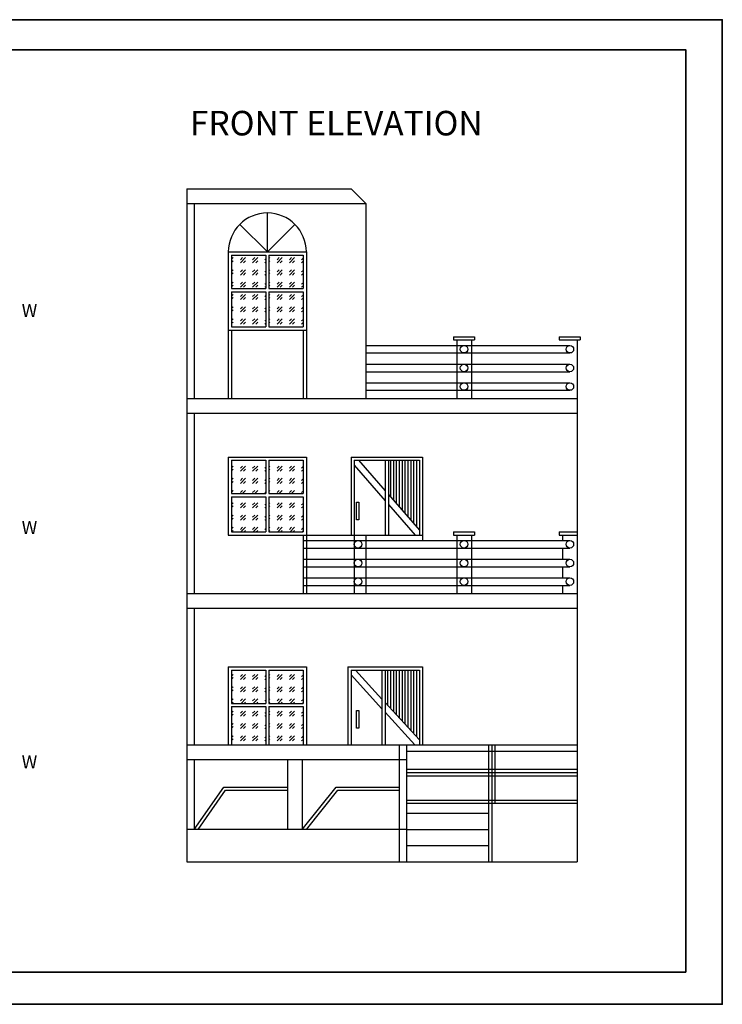
# Model space of a CAD drawing. Units: inches. Extents: x 28637 to 29820, y 17246 to 17928.
# Tile 6 of 6: x 29334 to 29820, y 17246 to 17928. Entities that reach past the tile are written whole.
import ezdxf

# ---------------------------------------------------------------- set-up
doc = ezdxf.new("R2010")
doc.units = ezdxf.units.IN
for name, color, linetype, lineweight in [('A-ANNO-TEXT', 7, 'Continuous', 25), ('A-ANNO-TTLB', 7, 'Continuous', 35), ('A-ELEV', 7, 'Continuous', 25), ('A-ELEV-PATT', 8, 'Continuous', 13)]:
    doc.layers.add(name, color=color, linetype=linetype, lineweight=lineweight)
doc.styles.get("Standard").update_dxf_attribs({"font": 'arial.ttf'})

msp = doc.modelspace()

# ---------------------------------------------------------------- hatches: boundary and pattern name
at = {"layer": 'A-ELEV-PATT'}
h = msp.add_hatch(dxfattribs=at)
h.set_pattern_fill('GOST_GLASS', color=256)
h.paths.add_polyline_path([(29503.9, 17764.93), (29480.27, 17764.93), (29480.27, 17741.85), (29503.9, 17741.85)])
h.paths.add_polyline_path([(29529.79, 17764.93), (29506.15, 17764.93), (29506.15, 17741.85), (29529.79, 17741.85)])
h.paths.add_polyline_path([(29503.9, 17739.6), (29480.27, 17739.6), (29480.27, 17715.4), (29503.9, 17715.4)])
h.paths.add_polyline_path([(29529.79, 17739.6), (29506.15, 17739.6), (29506.15, 17715.4), (29529.79, 17715.4)])
h.paths.add_polyline_path([(29503.9, 17622.97), (29480.27, 17622.97), (29480.27, 17599.9), (29503.9, 17599.9)])
h.paths.add_polyline_path([(29529.79, 17622.97), (29506.15, 17622.97), (29506.15, 17599.9), (29529.79, 17599.9)])
h.paths.add_polyline_path([(29503.9, 17597.65), (29480.27, 17597.65), (29480.27, 17573.45), (29503.9, 17573.45)])
h.paths.add_polyline_path([(29529.79, 17597.65), (29506.15, 17597.65), (29506.15, 17573.45), (29529.79, 17573.45)])
h.paths.add_polyline_path([(29503.9, 17477.79), (29480.27, 17477.79), (29480.27, 17454.71), (29503.9, 17454.71)])
h.paths.add_polyline_path([(29529.79, 17477.79), (29506.15, 17477.79), (29506.15, 17454.71), (29529.79, 17454.71)])
h.paths.add_polyline_path([(29503.9, 17452.46), (29480.27, 17452.46), (29480.27, 17427.14), (29480.27, 17426.01), (29529.79, 17426.01), (29529.79, 17452.46), (29506.15, 17452.46), (29506.15, 17427.14), (29503.9, 17427.14)])

# ---------------------------------------------------------------- linework, layer by layer
at = {"layer": 'A-ANNO-TTLB'}
for points in [[(28637.03, 17927.97), (29820.02, 17927.97), (29820.02, 17246.37), (28637.03, 17246.37)], [(28663.78, 17907.18), (29794.75, 17907.18), (29794.75, 17268.65), (28663.78, 17268.65)]]:
    msp.add_lwpolyline(points, close=True, dxfattribs=at)
at = {"layer": 'A-ELEV'}
for p, q in [((29449.31, 17810.93), (29562.99, 17810.93)), ((29449.31, 17810.93), (29449.31, 17800.8)), ((29562.99, 17810.93), (29573.12, 17800.8)), ((29449.31, 17800.8), (29449.31, 17344.98)), ((29449.31, 17800.8), (29562.99, 17800.8)), ((29454.38, 17800.8), (29454.38, 17665.74)), ((29562.99, 17800.8), (29573.12, 17800.8)), ((29573.12, 17800.8), (29573.12, 17706.26)), ((29505.03, 17767.18), (29505.03, 17794.19)), ((29505.03, 17767.18), (29485.92, 17786.27)), ((29505.03, 17767.18), (29524.13, 17786.27)), ((29478.01, 17767.18), (29478.01, 17665.74)), ((29478.01, 17767.18), (29532.04, 17767.18)), ((29478.01, 17767.18), (29532.04, 17767.18)), ((29480.27, 17764.93), (29480.27, 17741.85)), ((29480.27, 17764.93), (29503.9, 17764.93)), ((29503.9, 17764.93), (29503.9, 17741.85)), ((29506.15, 17764.93), (29506.15, 17741.85)), ((29506.15, 17764.93), (29529.79, 17764.93)), ((29529.79, 17764.93), (29529.79, 17741.85)), ((29532.04, 17767.18), (29532.04, 17665.74)), ((29532.04, 17767.18), (29532.04, 17665.74)), ((29480.27, 17741.85), (29503.9, 17741.85)), ((29480.27, 17739.6), (29503.9, 17739.6)), ((29480.27, 17739.6), (29480.27, 17715.4)), ((29503.9, 17739.6), (29503.9, 17715.4)), ((29506.15, 17741.85), (29529.79, 17741.85)), ((29506.15, 17739.6), (29506.15, 17715.4)), ((29506.15, 17739.6), (29529.79, 17739.6)), ((29529.79, 17739.6), (29529.79, 17715.4)), ((29480.27, 17715.4), (29503.9, 17715.4)), ((29506.15, 17715.4), (29529.79, 17715.4)), ((29478.01, 17713.15), (29532.04, 17713.15)), ((29480.27, 17713.15), (29480.27, 17665.74)), ((29529.79, 17713.15), (29529.79, 17665.74)), ((29633.89, 17708.51), (29648.53, 17708.51)), ((29633.89, 17708.51), (29633.89, 17706.26)), ((29648.53, 17708.51), (29648.53, 17706.26)), ((29707.05, 17708.51), (29721.68, 17708.51)), ((29707.05, 17708.51), (29707.05, 17706.26)), ((29721.68, 17708.51), (29721.68, 17706.26)), ((29573.12, 17706.26), (29573.12, 17665.74)), ((29573.12, 17702.41), (29714.46, 17702.41)), ((29633.89, 17706.26), (29648.53, 17706.26)), ((29636.15, 17706.26), (29636.15, 17665.74)), ((29646.28, 17706.26), (29646.28, 17665.74)), ((29707.05, 17706.26), (29721.68, 17706.26)), ((29719.43, 17706.26), (29719.43, 17344.98)), ((29573.12, 17697.26), (29714.46, 17697.26)), ((29573.12, 17689.5), (29714.46, 17689.5)), ((29573.12, 17684.24), (29714.46, 17684.24)), ((29573.12, 17676.64), (29714.46, 17676.64)), ((29573.12, 17671.42), (29714.46, 17671.42)), ((29449.31, 17665.74), (29719.43, 17665.74)), ((29449.31, 17655.61), (29719.43, 17655.61)), ((29454.38, 17655.61), (29454.38, 17530.68)), ((29478.01, 17625.23), (29532.04, 17625.23)), ((29478.01, 17625.23), (29478.01, 17571.2)), ((29480.27, 17622.97), (29503.9, 17622.97)), ((29480.27, 17622.97), (29480.27, 17599.9)), ((29503.9, 17622.97), (29503.9, 17599.9)), ((29506.15, 17622.97), (29506.15, 17599.9)), ((29506.15, 17622.97), (29529.79, 17622.97)), ((29529.79, 17622.97), (29529.79, 17599.9)), ((29532.04, 17625.23), (29532.04, 17530.68)), ((29562.99, 17625.23), (29612.51, 17625.23)), ((29562.99, 17625.23), (29562.99, 17571.2)), ((29565.24, 17622.97), (29565.24, 17571.2)), ((29565.24, 17622.97), (29610.26, 17622.97)), ((29565.24, 17619.54), (29586.62, 17594.95)), ((29568.22, 17622.97), (29586.62, 17601.81)), ((29586.62, 17622.97), (29586.62, 17571.2)), ((29588.88, 17622.97), (29588.88, 17571.2)), ((29590.26, 17622.97), (29590.26, 17597.63)), ((29592.26, 17622.97), (29592.26, 17595.33)), ((29594.26, 17622.97), (29594.26, 17593.03)), ((29596.26, 17622.97), (29596.26, 17590.73)), ((29598.26, 17622.97), (29598.26, 17588.43)), ((29600.26, 17622.97), (29600.26, 17586.13)), ((29602.26, 17622.97), (29602.26, 17583.83)), ((29604.26, 17622.97), (29604.26, 17581.53)), ((29606.26, 17622.97), (29606.26, 17579.23)), ((29608.26, 17622.97), (29608.26, 17576.93)), ((29610.26, 17622.97), (29610.26, 17571.2)), ((29612.51, 17625.23), (29612.51, 17567.38)), ((29480.27, 17599.9), (29503.9, 17599.9)), ((29506.15, 17599.9), (29529.79, 17599.9)), ((29588.88, 17599.22), (29610.26, 17574.63)), ((29480.27, 17597.65), (29503.9, 17597.65)), ((29480.27, 17597.65), (29480.27, 17573.45)), ((29503.9, 17597.65), (29503.9, 17573.45)), ((29506.15, 17597.65), (29529.79, 17597.65)), ((29506.15, 17597.65), (29506.15, 17573.45)), ((29529.79, 17597.65), (29529.79, 17573.45)), ((29588.88, 17592.36), (29607.28, 17571.2)), ((29480.27, 17573.45), (29503.9, 17573.45)), ((29506.15, 17573.45), (29529.79, 17573.45)), ((29633.89, 17573.48), (29648.53, 17573.48)), ((29633.89, 17573.48), (29633.89, 17571.23)), ((29648.53, 17573.48), (29648.53, 17571.23)), ((29707.05, 17573.48), (29707.05, 17571.23)), ((29707.05, 17573.48), (29719.43, 17573.48)), ((29478.01, 17571.2), (29532.04, 17571.2)), ((29478.01, 17571.2), (29612.51, 17571.2)), ((29529.79, 17571.2), (29529.79, 17530.68)), ((29529.79, 17567.38), (29714.46, 17567.38)), ((29565.24, 17571.2), (29565.24, 17530.68)), ((29573.12, 17571.23), (29573.12, 17530.71)), ((29633.89, 17571.23), (29648.53, 17571.23)), ((29636.15, 17571.23), (29636.15, 17530.71)), ((29636.15, 17571.2), (29646.28, 17571.2)), ((29646.28, 17571.23), (29646.28, 17530.71)), ((29707.05, 17571.23), (29719.43, 17571.23)), ((29709.3, 17571.23), (29709.3, 17567.38)), ((29709.3, 17571.2), (29719.43, 17571.2)), ((29529.79, 17562.22), (29714.46, 17562.22)), ((29709.3, 17562.22), (29709.3, 17554.46)), ((29529.79, 17554.46), (29714.46, 17554.46)), ((29529.79, 17549.2), (29714.46, 17549.2)), ((29709.3, 17549.2), (29709.3, 17541.61)), ((29529.79, 17541.61), (29714.46, 17541.61)), ((29529.79, 17536.38), (29714.46, 17536.38)), ((29709.3, 17536.38), (29709.3, 17530.68)), ((29449.31, 17530.68), (29719.43, 17530.68)), ((29449.31, 17520.56), (29719.43, 17520.56)), ((29454.38, 17520.56), (29454.38, 17426.01)), ((29478.01, 17480.04), (29532.04, 17480.04)), ((29478.01, 17480.04), (29478.01, 17426.01)), ((29478.01, 17480.04), (29478.01, 17426.01)), ((29480.27, 17477.79), (29503.9, 17477.79)), ((29480.27, 17477.79), (29480.27, 17454.71)), ((29480.27, 17477.79), (29480.27, 17454.71)), ((29503.9, 17477.79), (29503.9, 17454.71)), ((29506.15, 17477.79), (29506.15, 17454.71)), ((29506.15, 17477.79), (29529.79, 17477.79)), ((29529.79, 17477.79), (29529.79, 17454.71)), ((29529.79, 17477.79), (29529.79, 17454.71)), ((29532.04, 17480.04), (29532.04, 17426.01)), ((29532.04, 17480.04), (29532.04, 17426.01)), ((29560.74, 17480.04), (29612.51, 17480.04)), ((29560.74, 17480.04), (29560.74, 17426.01)), ((29562.99, 17477.79), (29562.99, 17426.01)), ((29562.99, 17477.79), (29610.26, 17477.79)), ((29566.04, 17477.79), (29584.37, 17457.7)), ((29584.37, 17477.79), (29584.37, 17426.01)), ((29586.62, 17477.79), (29586.62, 17426.01)), ((29588.26, 17477.79), (29588.26, 17453.45)), ((29590.26, 17477.79), (29590.26, 17451.26)), ((29592.26, 17477.79), (29592.26, 17449.07)), ((29594.26, 17477.79), (29594.26, 17446.88)), ((29596.26, 17477.79), (29596.26, 17444.69)), ((29598.26, 17477.79), (29598.26, 17442.5)), ((29600.26, 17477.79), (29600.26, 17440.3)), ((29602.26, 17477.79), (29602.26, 17438.11)), ((29604.26, 17477.79), (29604.26, 17435.92)), ((29606.26, 17477.79), (29606.26, 17433.73)), ((29608.26, 17477.79), (29608.26, 17431.54)), ((29610.26, 17477.79), (29610.26, 17426.01)), ((29612.51, 17480.04), (29612.51, 17426.01)), ((29562.99, 17474.45), (29584.37, 17451.03)), ((29480.27, 17454.71), (29503.9, 17454.71)), ((29480.27, 17452.46), (29503.9, 17452.46)), ((29480.27, 17452.46), (29480.27, 17427.14)), ((29480.27, 17452.46), (29480.27, 17426.01)), ((29503.9, 17452.46), (29503.9, 17426.01)), ((29506.15, 17454.71), (29529.79, 17454.71)), ((29506.15, 17452.46), (29529.79, 17452.46)), ((29506.15, 17452.46), (29506.15, 17426.01)), ((29529.79, 17452.46), (29529.79, 17426.01)), ((29529.79, 17452.46), (29529.79, 17426.01)), ((29586.62, 17455.24), (29610.26, 17429.35)), ((29586.62, 17448.56), (29607.21, 17426.01)), ((29449.31, 17426.01), (29562.99, 17426.01)), ((29478.01, 17426.01), (29532.04, 17426.01)), ((29562.99, 17426.01), (29601.26, 17426.01)), ((29596.19, 17426.01), (29596.19, 17344.98)), ((29601.26, 17426.01), (29719.43, 17426.01)), ((29601.26, 17426.01), (29601.26, 17344.98)), ((29658.09, 17426.01), (29658.09, 17385.5)), ((29658.09, 17426.01), (29658.09, 17344.98)), ((29660.34, 17426.01), (29660.34, 17344.98)), ((29662.59, 17426.01), (29662.59, 17385.5)), ((29449.31, 17415.88), (29601.26, 17415.88)), ((29454.38, 17415.88), (29454.38, 17367.49)), ((29519.09, 17415.88), (29519.09, 17367.49)), ((29529.22, 17415.88), (29529.22, 17367.49)), ((29601.26, 17421.51), (29719.43, 17421.51)), ((29601.26, 17409.13), (29719.43, 17409.13)), ((29601.26, 17406.88), (29719.43, 17406.88)), ((29601.26, 17404.63), (29719.43, 17404.63)), ((29454.38, 17367.49), (29474.98, 17396.75)), ((29457.13, 17367.49), (29476.15, 17394.5)), ((29474.98, 17396.75), (29519.09, 17396.75)), ((29476.15, 17394.5), (29519.09, 17394.5)), ((29529.22, 17367.49), (29552.66, 17396.75)), ((29532.11, 17367.49), (29553.74, 17394.5)), ((29552.66, 17396.75), (29596.19, 17396.75)), ((29553.74, 17394.5), (29596.19, 17394.5)), ((29601.26, 17387.75), (29719.43, 17387.75)), ((29601.26, 17385.5), (29719.43, 17385.5)), ((29601.26, 17378.74), (29658.09, 17378.74)), ((29601.26, 17367.49), (29449.31, 17367.49)), ((29601.26, 17367.49), (29658.09, 17367.49)), ((29601.26, 17356.23), (29658.09, 17356.23)), ((29449.31, 17344.98), (29719.43, 17344.98))]:
    msp.add_line(p, q, dxfattribs=at)
for points in [[(29566.8, 17593.93), (29568.32, 17593.93), (29568.32, 17581.69), (29566.8, 17581.69)], [(29566.8, 17449.8), (29568.32, 17449.8), (29568.32, 17437.57), (29566.8, 17437.57)]]:
    msp.add_lwpolyline(points, close=True, dxfattribs=at)
for centre in [(29641.19, 17699.85), (29714.49, 17699.85), (29641.19, 17686.86), (29714.49, 17686.86), (29641.19, 17674.02), (29714.49, 17674.02), (29567.85, 17564.81), (29641.19, 17564.81), (29714.49, 17564.81), (29567.85, 17551.82), (29641.19, 17551.82), (29714.49, 17551.82), (29567.85, 17538.99), (29641.19, 17538.99), (29714.49, 17538.99)]:
    msp.add_circle(centre, 2.6, dxfattribs=at)
msp.add_arc((29505.03, 17767.18), 27.01, 0, 180, dxfattribs=at)

# ---------------------------------------------------------------- texts
at = {"layer": 'A-ANNO-TEXT'}
for s, height, p in [('   FRONT ELEVATION', 17, (29435.86, 17847.85)), ('    W', 9, (29323.95, 17722.18)), ('    W', 9, (29323.95, 17571.93)), ('    W', 9, (29323.95, 17409.66))]:
    msp.add_text(s, height=height, dxfattribs=at).set_placement(p)

doc.saveas('drawing.dxf')
